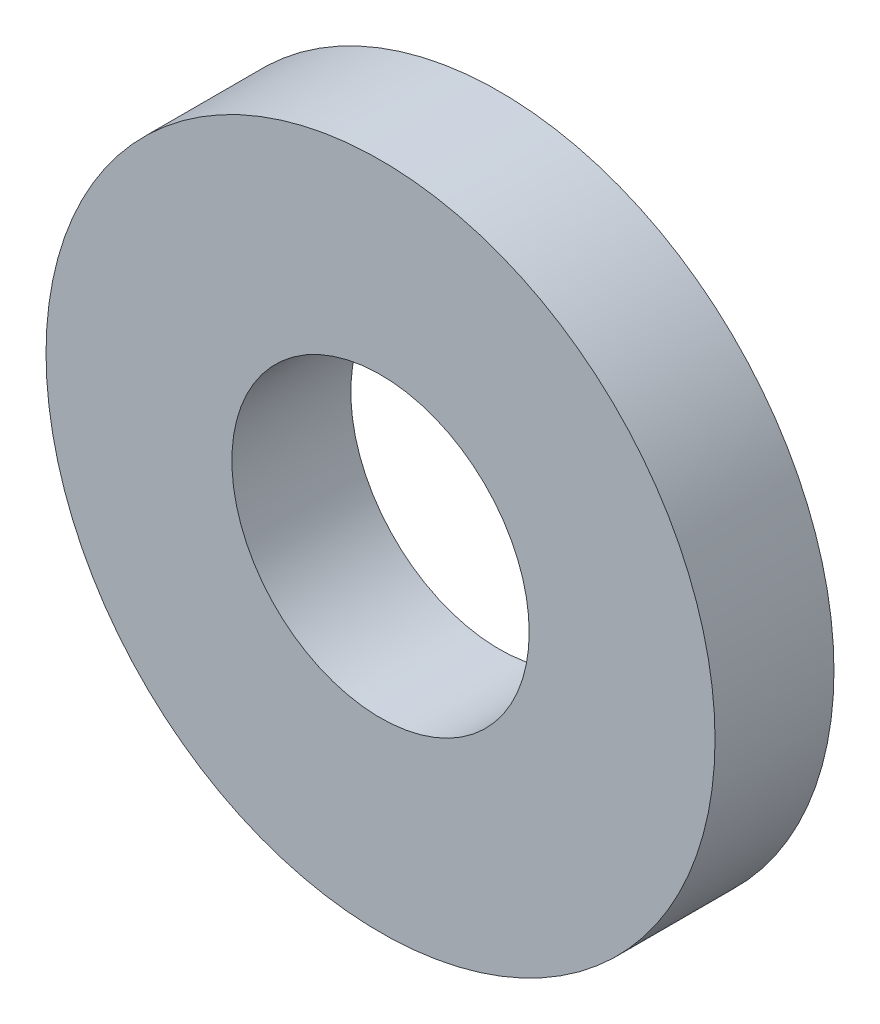
from build123d import *

# Parameters (mm, degrees)
WASHER_PROFILE_45_20_R   = 22.5
WASHER_PROFILE_45_20_R_2 = 10
WASHER_BODY_8MM_DEPTH    = 8


with BuildPart() as part:
    # Washer Profile Ø45-Ø20 → Washer Body 8mm (new body)
    with BuildSketch(Plane.XY):
        Circle(WASHER_PROFILE_45_20_R)
        Circle(WASHER_PROFILE_45_20_R_2, mode=Mode.SUBTRACT)
    extrude(amount=WASHER_BODY_8MM_DEPTH)


solid = part.part
